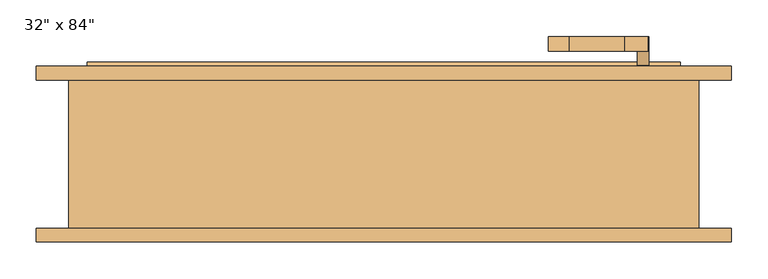
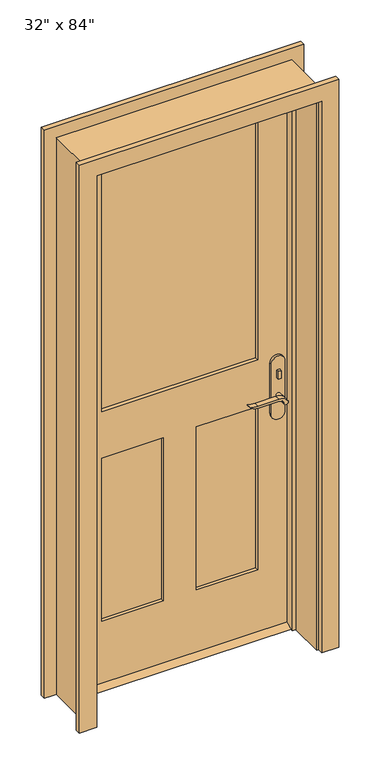
"""IFC4 building model written with IfcOpenShell, lengths in millimetres: door geometry."""

from ifc_helpers import new_model, si_unit, point, frame, frame_2d, origin, place, context, project, spatial, polyline, circle_curve, trimmed, segment, composite_curve, outline, extrude, faceted_brep, source, transform, mapped, element, save


def door_823c627a(model_context):
    return source(origin(), model_context, "Body", "SolidModel", [
        extrude(outline(polyline([(63.5, 12.7), (98.425, 12.7), (123.825, 0.0), (38.1, 0.0), (63.5, 12.7)])), frame((-406.4, 0.0, 0.0), z_axis=(1.0, 0.0, 0.0), x_axis=(0.0, 1.0, 0.0)), (0.0, 0.0, 1.0), 812.8),
        extrude(outline(polyline([(360.6, 43.5), (350.6, 43.5), (350.6, 53.5), (360.6, 53.5), (360.6, 43.5)])), frame((0.0, 0.0, 981.9), z_axis=(0.0, 0.0, 1.0), x_axis=(1.0, 0.0, 0.0)), (0.0, 0.0, 1.0), 30.0),
        extrude(outline(composite_curve([segment(trimmed(circle_curve(frame_2d((996.9, 355.6)), 8.0), [point((996.9, 347.6))], [point((996.9, 363.6))], False, "CARTESIAN"), True, "CONTINUOUS"), segment(trimmed(circle_curve(frame_2d((996.9, 355.6)), 8.0), [point((996.9, 363.6))], [point((996.9, 347.6))], False, "CARTESIAN"), True, "CONTINUOUS")], self_intersect=False)), frame((0.0, 108.425, 0.0), z_axis=(0.0, 1.0, 0.0), x_axis=(0.0, 0.0, 1.0)), (0.0, 0.0, 1.0), 10.0),
        extrude(outline(composite_curve([segment(trimmed(circle_curve(frame_2d((897.1555521, 331.9324871)), 37.2832219), [point((919.0523287, 362.1081363))], [point((934.4, 330.2325667))], False, "CARTESIAN"), True, "CONTINUOUS"), segment(polyline([(934.4, 330.2325667), (934.4, 253.9564091)]), True, "CONTINUOUS"), segment(trimmed(circle_curve(frame_2d((1017.6850638, 254.0227909)), 83.2850902), [point((934.4, 253.9564091))], [point((939.4, 225.6))], True, "CARTESIAN"), True, "CONTINUOUS"), segment(polyline([(939.4, 225.6), (936.6135558, 225.6)]), True, "CONTINUOUS"), segment(trimmed(circle_curve(frame_2d((986.6709207, 257.5396612)), 59.3791355), [point((936.6135558, 225.6))], [point((927.4, 253.9564091))], False, "CARTESIAN"), True, "CONTINUOUS"), segment(polyline([(927.4, 253.9564091), (927.4, 330.2138099)]), True, "CONTINUOUS"), segment(trimmed(circle_curve(frame_2d((909.2738613, 330.2138099)), 18.1261387), [point((927.4, 330.2138099))], [point((914.4, 347.6))], True, "CARTESIAN"), True, "CONTINUOUS"), segment(trimmed(circle_curve(frame_2d((914.4, 355.6)), 8.0), [point((914.4, 347.6))], [point((919.0523287, 362.1081363))], False, "CARTESIAN"), True, "CONTINUOUS")], self_intersect=False)), frame((0.0, 3.5, 0.0), z_axis=(0.0, 1.0, 0.0), x_axis=(0.0, 0.0, 1.0)), (0.0, 0.0, 1.0), 20.0),
        extrude(outline(composite_curve([segment(trimmed(circle_curve(frame_2d((914.4, 355.6)), 8.0), [point((914.3999903, 347.6))], [point((919.0523287, 362.1081363))], False, "CARTESIAN"), True, "CONTINUOUS"), segment(trimmed(circle_curve(frame_2d((897.1555521, 331.9324871)), 37.2832219), [point((919.0523287, 362.1081363))], [point((934.4, 330.2325667))], False, "CARTESIAN"), True, "CONTINUOUS"), segment(polyline([(934.4, 330.2325667), (934.4, 253.9564091)]), True, "CONTINUOUS"), segment(trimmed(circle_curve(frame_2d((1017.6850638, 254.0227909)), 83.2850902), [point((934.4, 253.9564091))], [point((939.4, 225.6))], True, "CARTESIAN"), True, "CONTINUOUS"), segment(polyline([(939.4, 225.6), (936.6135558, 225.6)]), True, "CONTINUOUS"), segment(trimmed(circle_curve(frame_2d((986.6709207, 257.5396612)), 59.3791355), [point((936.6135558, 225.6))], [point((927.4, 253.9564091))], False, "CARTESIAN"), True, "CONTINUOUS"), segment(polyline([(927.4, 253.9564091), (927.4, 330.2138122)]), True, "CONTINUOUS"), segment(trimmed(circle_curve(frame_2d((909.2738682, 330.2138122)), 18.1261318), [point((927.4, 330.2138122))], [point((914.3999903, 347.6))], True, "CARTESIAN"), True, "CONTINUOUS")], self_intersect=False)), frame((0.0, 138.425, 0.0), z_axis=(0.0, 1.0, 0.0), x_axis=(0.0, 0.0, 1.0)), (0.0, 0.0, 1.0), 20.0),
        extrude(outline(composite_curve([segment(trimmed(circle_curve(frame_2d((914.4, 355.6)), 8.0), [point((914.4, 347.6))], [point((914.4, 363.6))], False, "CARTESIAN"), True, "CONTINUOUS"), segment(trimmed(circle_curve(frame_2d((914.4, 355.6)), 8.0), [point((914.4, 363.6))], [point((914.4, 347.6))], False, "CARTESIAN"), True, "CONTINUOUS")], self_intersect=False)), frame((0.0, 23.5, 0.0), z_axis=(0.0, 1.0, 0.0), x_axis=(0.0, 0.0, 1.0)), (0.0, 0.0, 1.0), 30.0),
        extrude(outline(composite_curve([segment(trimmed(circle_curve(frame_2d((914.4, 355.6)), 8.0), [point((914.4, 347.6))], [point((914.4, 363.6))], False, "CARTESIAN"), True, "CONTINUOUS"), segment(trimmed(circle_curve(frame_2d((914.4, 355.6)), 8.0), [point((914.4, 363.6))], [point((914.4, 347.6))], False, "CARTESIAN"), True, "CONTINUOUS")], self_intersect=False)), frame((0.0, 108.425, 0.0), z_axis=(0.0, 1.0, 0.0), x_axis=(0.0, 0.0, 1.0)), (0.0, 0.0, 1.0), 30.0),
        extrude(outline(composite_curve([segment(polyline([(844.4, 380.6), (1039.4, 380.6)]), True, "CONTINUOUS"), segment(trimmed(circle_curve(frame_2d((1039.4, 355.6)), 25.0), [point((1039.4, 380.6))], [point((1039.4, 330.6))], False, "CARTESIAN"), True, "CONTINUOUS"), segment(polyline([(1039.4, 330.6), (844.4, 330.6)]), True, "CONTINUOUS"), segment(trimmed(circle_curve(frame_2d((844.4, 355.6)), 25.0), [point((844.4, 330.6))], [point((844.4, 380.6))], False, "CARTESIAN"), True, "CONTINUOUS")], self_intersect=False)), frame((0.0, 53.5, 0.0), z_axis=(0.0, 1.0, 0.0), x_axis=(0.0, 0.0, 1.0)), (0.0, 0.0, 1.0), 10.0),
        extrude(outline(composite_curve([segment(polyline([(844.4, 380.6), (1039.4, 380.6)]), True, "CONTINUOUS"), segment(trimmed(circle_curve(frame_2d((1039.4, 355.6)), 25.0), [point((1039.4, 380.6))], [point((1039.4, 330.6))], False, "CARTESIAN"), True, "CONTINUOUS"), segment(polyline([(1039.4, 330.6), (844.4, 330.6)]), True, "CONTINUOUS"), segment(trimmed(circle_curve(frame_2d((844.4, 355.6)), 25.0), [point((844.4, 330.6))], [point((844.4, 380.6))], False, "CARTESIAN"), True, "CONTINUOUS")], self_intersect=False)), frame((0.0, 98.425, 0.0), z_axis=(0.0, 1.0, 0.0), x_axis=(0.0, 0.0, 1.0)), (0.0, 0.0, 1.0), 10.0),
        extrude(outline(polyline([(2133.6, -406.4), (12.7, -406.4), (12.7, 406.4), (2133.6, 406.4), (2133.6, -406.4)]), holes=[polyline([(1066.8, -285.75), (2012.95, -285.75), (2012.95, 285.75), (1066.8, 285.75), (1066.8, -285.75)]), polyline([(885.825, -60.325), (254.0, -60.325), (254.0, -285.75), (885.825, -285.75), (885.825, -60.325)]), polyline([(885.825, 285.75), (254.0, 285.75), (254.0, 60.325), (885.825, 60.325), (885.825, 285.75)])]), frame((0.0, 63.5, 0.0), z_axis=(0.0, 1.0, 0.0), x_axis=(0.0, 0.0, 1.0)), (0.0, 0.0, 1.0), 34.925),
        faceted_brep([(431.8, 98.425, 0.0), (431.8, -104.775, 0.0), (406.4, -104.775, 0.0), (406.4, 28.575, 0.0), (393.7, 28.575, 0.0), (393.7, 63.5, 0.0), (406.4, 63.5, 0.0), (406.4, 98.425, 0.0), (431.8, 98.425, 2159.0), (431.8, -104.775, 2159.0), (-431.8, -104.775, 2159.0), (-431.8, -104.775, 0.0), (-406.4, -104.775, 0.0), (-406.4, -104.775, 2133.6), (406.4, -104.775, 2133.6), (406.4, 28.575, 2133.6), (-406.4, 28.575, 2133.6), (-406.4, 28.575, 0.0), (-393.7, 28.575, 0.0), (-393.7, 28.575, 2120.9), (393.7, 28.575, 2120.9), (393.7, 63.5, 2120.9), (-393.7, 63.5, 2120.9), (-393.7, 63.5, 0.0), (-406.4, 63.5, 0.0), (-406.4, 63.5, 2133.6), (406.4, 63.5, 2133.6), (406.4, 98.425, 2133.6), (-406.4, 98.425, 2133.6), (-406.4, 98.425, 0.0), (-431.8, 98.425, 0.0), (-431.8, 98.425, 2159.0)], [[[0, 1, 2, 3, 4, 5, 6, 7]], [[1, 0, 8, 9]], [[2, 1, 9, 10, 11, 12, 13, 14]], [[3, 2, 14, 15]], [[4, 3, 15, 16, 17, 18, 19, 20]], [[5, 4, 20, 21]], [[6, 5, 21, 22, 23, 24, 25, 26]], [[7, 6, 26, 27]], [[0, 7, 27, 28, 29, 30, 31, 8]], [[9, 8, 31, 10]], [[15, 14, 13, 16]], [[21, 20, 19, 22]], [[27, 26, 25, 28]], [[30, 29, 24, 23, 18, 17, 12, 11]], [[10, 31, 30, 11]], [[16, 13, 12, 17]], [[22, 19, 18, 23]], [[28, 25, 24, 29]]]),
        extrude(outline(polyline([(-60.325, 75.1416667), (-285.75, 75.1416667), (-285.75, 86.7833333), (-60.325, 86.7833333), (-60.325, 75.1416667)])), frame((0.0, 0.0, 254.0), z_axis=(0.0, 0.0, 1.0), x_axis=(1.0, 0.0, 0.0)), (0.0, 0.0, 1.0), 631.825),
        extrude(outline(polyline([(285.75, 75.1416667), (60.325, 75.1416667), (60.325, 86.7833333), (285.75, 86.7833333), (285.75, 75.1416667)])), frame((0.0, 0.0, 254.0), z_axis=(0.0, 0.0, 1.0), x_axis=(1.0, 0.0, 0.0)), (0.0, 0.0, 1.0), 631.825),
        extrude(outline(polyline([(285.75, 77.47), (-285.75, 77.47), (-285.75, 84.455), (285.75, 84.455), (285.75, 77.47)])), frame((0.0, 0.0, 1066.8), z_axis=(0.0, 0.0, 1.0), x_axis=(1.0, 0.0, 0.0)), (0.0, 0.0, 1.0), 946.15),
        extrude(outline(polyline([(0.0, -476.25), (0.0, -412.75), (2139.95, -412.75), (2139.95, 412.75), (0.0, 412.75), (0.0, 476.25), (2203.45, 476.25), (2203.45, -476.25), (0.0, -476.25)])), frame((0.0, -123.825, 0.0), z_axis=(0.0, 1.0, 0.0), x_axis=(0.0, 0.0, 1.0)), (0.0, 0.0, 1.0), 19.05),
        extrude(outline(polyline([(0.0, -476.25), (0.0, -412.75), (2139.95, -412.75), (2139.95, 412.75), (0.0, 412.75), (0.0, 476.25), (2203.45, 476.25), (2203.45, -476.25), (0.0, -476.25)])), frame((0.0, 98.425, 0.0), z_axis=(0.0, 1.0, 0.0), x_axis=(0.0, 0.0, 1.0)), (0.0, 0.0, 1.0), 19.05),
    ])


if __name__ == "__main__":
    model = new_model("IFC4")
    model_context = context("Model", 3, world=origin())
    ifc_project = project(units=[si_unit("LENGTHUNIT", "METRE", prefix="MILLI")], contexts=[model_context])
    site = spatial("IfcSite", under=ifc_project)
    building = spatial("IfcBuilding", under=site)
    placement = place(None, origin())
    door_shape = door_823c627a(model_context)
    element("IfcDoor", 1, ObjectType="32\" x 84\"", at=placement, inside=building, context=model_context, shape_type="MappedRepresentation", body=[
        mapped(door_shape, transform((0.0, 0.0, 0.0), x_axis=(1.0, 0.0, 0.0), y_axis=(0.0, 1.0, 0.0), z_axis=(0.0, 0.0, 1.0))),
    ])
    save(model, "model.ifc")

# Revit data of these elements
# Type "32\" x 84\""
#   Type Mark = "15"
#   Assembly Code = "B2030100"
#   Analytic Construction = "French door, wood frame with single glass"
#   Top Rail = 0' - 4 3/4"
#   Threshold Offset [instance default] = 0' - 0 1/2"
#   Thickness = 0' - 1 3/8"
#   Thermal Resistance (R) = 1.0696 (h·ft²·°F)/BTU
#   Swing Angle [instance default] = 90.00°
#   Stiles = 0' - 4 3/4"
#   Rough Width = 2' - 10"
#   Rough Height = 7' - 1"
#   Lock Rail = 0' - 7 1/8"
#   Height = 7' - 0"
#   Width = 2' - 8"
#   Heat Transfer Coefficient (U) = 0.9350 BTU/(h·ft²·°F)
#   Door Offset [instance default] = 0' - 0"
#   Bottom Rail = 0' - 9 1/2"
#   Threshold [instance default] = yes
#   Function = 1
#   Exterior Trim [instance default] = yes
#   Trim Material = Cherry
#   Threshold Material = Cherry
#   Panel Material = Cherry
#   Glazing = Glass
#   Frame Material = Cherry
#   Door Handle Material = Aluminum
#   Visual Light Transmittance = 0
#   Solar Heat Gain Coefficient = 0
#   Wall Closure = (empty or 0)
#   Construction Type = (empty or 0)
# Element 1 (IfcDoor, "32\" x 84\"")
#   Materials on its faces: "Cherry", "Aluminum", "Glass"
# Materials
#   "Cherry": class "Wood", colour RGB 226 177 128, transparency 0, Description = "Prunus Serotina", Cost = 0
#   "Glass": class "Glass", colour RGB 0 128 192, transparency 0.75, Description = "Soda Lime Glass", Cost = 0
#   "Aluminum": class "Metal", colour RGB 247 247 247, transparency 0, Description = "Aluminum 6061", Cost = 0
